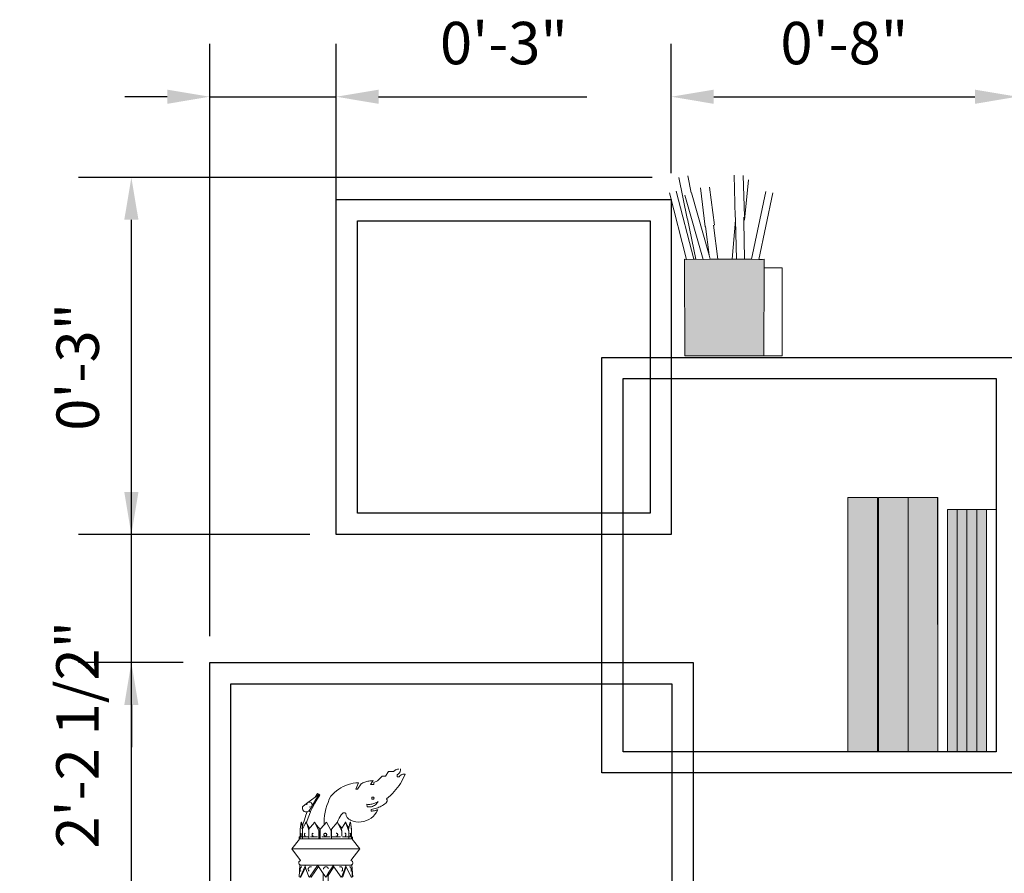
# Model space of a CAD drawing. Units: millimetres. Extents: x 7894 to 8038, y 6851 to 6951.
# Tile 6 of 49: x 7940.01 to 7963.22, y 6871.49 to 6891.62. Entities that reach past the tile are written whole.
import ezdxf

# ---------------------------------------------------------------- set-up
doc = ezdxf.new("R2010")
doc.units = ezdxf.units.MM
for name, color, linetype, lineweight in [('A-ANNO-DIMS', 2, 'Continuous', 18), ('A-FURN-ACCS', 8, 'Continuous', 13), ('A-FURN-BOOK', 8, 'Continuous', 13), ('A-FURN-CASE', 7, 'Continuous', 30)]:
    doc.layers.add(name, color=color, linetype=linetype, lineweight=lineweight)
doc.layers.add('A-FURN-ACCS-PATT', color=116, linetype='Continuous', lineweight=9, true_color=0x136734)
doc.layers.add('A-FURN-PATT', color=32, linetype='Continuous', lineweight=9, true_color=0xcd6928)
doc.styles.get("Standard").update_dxf_attribs({"font": 'arial.ttf'})
doc.dimstyles.new('ISO-25', dxfattribs={"dimtxt": 1, "dimasz": 1, "dimexe": 1.25, "dimexo": 0.625, "dimtad": 1, "dimdec": 0, "dimlunit": 4, "dimtxsty": 'Standard', "dimcen": 2.5, "dimclrt": 1, "dimadec": 0, "dimazin": 0, "dimtfac": 1, "dimtdec": 0, "dimtmove": 0, "dimatfit": 3, "dimfxl": 1, "dimarcsym": 0})

# ---------------------------------------------------------------- blocks, each defined once
blk = doc.blocks.new('DISPLAY-LEAF-FINIAL')
for p, q in [((2.447, 3.478), (2.461, 3.485)), ((2.461, 3.485), (2.475, 3.491)), ((2.475, 3.491), (2.489, 3.496)), ((2.489, 3.496), (2.504, 3.501)), ((2.504, 3.501), (2.519, 3.504)), ((2.565, 3.494), (2.563, 3.479)), ((2.565, 3.508), (2.565, 3.494)), ((2.023, 3.221), (2.127, 3.334)), ((2.127, 3.334), (2.209, 3.334)), ((2.209, 3.334), (2.276, 3.441)), ((2.276, 3.441), (2.398, 3.441)), ((2.398, 3.441), (2.409, 3.452)), ((2.409, 3.452), (2.421, 3.461)), ((2.421, 3.461), (2.434, 3.47)), ((2.434, 3.47), (2.447, 3.478)), ((2.493, 3.371), (2.48, 3.364)), ((2.48, 3.364), (2.48, 3.316)), ((2.48, 3.316), (2.533, 3.316)), ((2.505, 3.379), (2.493, 3.371)), ((2.516, 3.389), (2.505, 3.379)), ((2.527, 3.4), (2.516, 3.389)), ((2.536, 3.411), (2.527, 3.4)), ((2.533, 3.316), (2.54, 3.327)), ((2.544, 3.424), (2.536, 3.411)), ((2.54, 3.327), (2.549, 3.338)), ((2.551, 3.437), (2.544, 3.424)), ((2.549, 3.338), (2.558, 3.347)), ((2.556, 3.45), (2.551, 3.437)), ((2.56, 3.465), (2.556, 3.45)), ((2.558, 3.347), (2.569, 3.356)), ((2.563, 3.479), (2.56, 3.465)), ((2.569, 3.356), (2.58, 3.363)), ((2.58, 3.363), (2.592, 3.37)), ((2.62, 3.27), (2.591, 3.216)), ((2.592, 3.37), (2.604, 3.375)), ((2.604, 3.375), (2.617, 3.379)), ((2.617, 3.379), (2.63, 3.382)), ((2.646, 3.325), (2.62, 3.27)), ((2.63, 3.382), (2.643, 3.383)), ((2.643, 3.383), (2.657, 3.383)), ((2.67, 3.382), (2.646, 3.325)), ((2.657, 3.383), (2.67, 3.382)), ((1.055, 2.986), (1.105, 3.023)), ((1.105, 3.023), (1.158, 3.056)), ((1.158, 3.056), (1.213, 3.085)), ((1.213, 3.085), (1.27, 3.111)), ((1.27, 3.111), (1.328, 3.133)), ((1.328, 3.133), (1.388, 3.15)), ((1.388, 3.15), (1.449, 3.164)), ((1.449, 3.164), (1.51, 3.173)), ((1.51, 3.173), (1.572, 3.179)), ((1.572, 3.179), (1.511, 3.024)), ((1.511, 3.024), (1.55, 3.024)), ((1.55, 3.024), (1.632, 3.152)), ((1.632, 3.152), (1.654, 3.163)), ((1.654, 3.163), (1.676, 3.173)), ((1.676, 3.173), (1.699, 3.182)), ((1.699, 3.182), (1.722, 3.191)), ((1.722, 3.191), (1.745, 3.198)), ((1.745, 3.198), (1.769, 3.205)), ((1.769, 3.205), (1.793, 3.211)), ((1.793, 3.211), (1.817, 3.216)), ((1.817, 3.216), (1.841, 3.22)), ((1.841, 3.22), (1.865, 3.223)), ((1.914, 3.227), (1.854, 3.133)), ((1.854, 3.133), (1.934, 3.133)), ((1.865, 3.223), (1.889, 3.226)), ((1.889, 3.226), (1.914, 3.227)), ((1.934, 3.185), (2.023, 3.221)), ((1.934, 3.133), (1.934, 3.185)), ((2.491, 3.062), (2.453, 3.014)), ((2.527, 3.112), (2.491, 3.062)), ((2.56, 3.163), (2.527, 3.112)), ((2.591, 3.216), (2.56, 3.163)), ((0.547, 2.84), (0.379, 2.713)), ((0.634, 2.9), (0.463, 2.609)), ((0.541, 2.696), (0.599, 2.791)), ((0.605, 2.924), (0.547, 2.84)), ((0.634, 2.905), (0.547, 2.84)), ((0.599, 2.791), (0.663, 2.885)), ((0.634, 2.905), (0.605, 2.924)), ((0.634, 2.9), (0.634, 2.905)), ((0.663, 2.885), (0.634, 2.905)), ((0.884, 2.786), (0.853, 2.713)), ((0.92, 2.857), (0.884, 2.786)), ((0.92, 2.857), (0.962, 2.903)), ((0.962, 2.903), (1.007, 2.946)), ((1.007, 2.946), (1.055, 2.986)), ((1.883, 2.817), (1.885, 2.824)), ((1.883, 2.81), (1.883, 2.817)), ((1.885, 2.803), (1.883, 2.81)), ((1.885, 2.824), (1.889, 2.831)), ((1.888, 2.797), (1.885, 2.803)), ((1.894, 2.791), (1.888, 2.797)), ((1.889, 2.831), (1.894, 2.836)), ((1.894, 2.836), (1.9, 2.839)), ((1.9, 2.788), (1.894, 2.791)), ((1.9, 2.839), (1.907, 2.841)), ((1.907, 2.786), (1.9, 2.788)), ((1.907, 2.841), (1.914, 2.841)), ((1.914, 2.841), (1.921, 2.839)), ((1.921, 2.788), (1.914, 2.786)), ((1.921, 2.839), (1.928, 2.836)), ((1.928, 2.791), (1.921, 2.788)), ((1.928, 2.836), (1.933, 2.83)), ((1.933, 2.796), (1.928, 2.791)), ((1.933, 2.83), (1.937, 2.824)), ((1.936, 2.803), (1.933, 2.796)), ((1.938, 2.81), (1.936, 2.803)), ((1.937, 2.824), (1.938, 2.817)), ((1.938, 2.817), (1.938, 2.81)), ((2.281, 2.839), (2.233, 2.801)), ((2.233, 2.801), (2.238, 2.792)), ((2.238, 2.792), (2.242, 2.783)), ((2.327, 2.88), (2.281, 2.839)), ((2.371, 2.923), (2.327, 2.88)), ((2.413, 2.967), (2.371, 2.923)), ((2.453, 3.014), (2.413, 2.967)), ((0.253, 2.607), (0.249, 2.584)), ((0.249, 2.58), (0.249, 2.584)), ((0.249, 2.58), (0.251, 2.557)), ((0.251, 2.557), (0.259, 2.536)), ((0.264, 2.627), (0.253, 2.607)), ((0.379, 2.713), (0.264, 2.627)), ((0.353, 2.675), (0.358, 2.69)), ((0.353, 2.66), (0.353, 2.675)), ((0.353, 2.659), (0.353, 2.66)), ((0.353, 2.657), (0.353, 2.659)), ((0.358, 2.69), (0.367, 2.703)), ((0.367, 2.703), (0.379, 2.713)), ((0.379, 2.713), (0.393, 2.72)), ((0.393, 2.72), (0.409, 2.723)), ((0.409, 2.723), (0.425, 2.722)), ((0.414, 2.606), (0.413, 2.603)), ((0.461, 2.605), (0.415, 2.527)), ((0.425, 2.722), (0.44, 2.718)), ((0.44, 2.718), (0.453, 2.709)), ((0.44, 2.496), (0.486, 2.593)), ((0.443, 2.613), (0.446, 2.612)), ((0.451, 2.615), (0.449, 2.616)), ((0.453, 2.709), (0.464, 2.698)), ((0.463, 2.609), (0.461, 2.605)), ((0.486, 2.593), (0.461, 2.605)), ((0.463, 2.609), (0.488, 2.597)), ((0.464, 2.698), (0.471, 2.684)), ((0.471, 2.684), (0.475, 2.669)), ((0.474, 2.667), (0.475, 2.669)), ((0.474, 2.667), (0.475, 2.666)), ((0.541, 2.696), (0.488, 2.597)), ((0.804, 2.562), (0.787, 2.485)), ((0.826, 2.638), (0.804, 2.562)), ((0.853, 2.713), (0.826, 2.638)), ((1.793, 2.668), (1.77, 2.67)), ((1.77, 2.67), (1.776, 2.611)), ((1.801, 2.608), (1.776, 2.611)), ((1.816, 2.667), (1.793, 2.668)), ((1.827, 2.607), (1.801, 2.608)), ((1.84, 2.668), (1.816, 2.667)), ((1.852, 2.609), (1.827, 2.607)), ((1.863, 2.67), (1.84, 2.668)), ((1.878, 2.613), (1.852, 2.609)), ((1.886, 2.673), (1.863, 2.67)), ((1.902, 2.62), (1.878, 2.613)), ((1.909, 2.678), (1.886, 2.673)), ((1.926, 2.63), (1.902, 2.62)), ((1.934, 2.561), (1.903, 2.554)), ((1.914, 2.786), (1.907, 2.786)), ((1.931, 2.684), (1.909, 2.678)), ((1.949, 2.642), (1.926, 2.63)), ((1.954, 2.692), (1.931, 2.684)), ((1.964, 2.569), (1.934, 2.561)), ((1.97, 2.657), (1.949, 2.642)), ((1.975, 2.701), (1.954, 2.692)), ((1.994, 2.578), (1.964, 2.569)), ((1.99, 2.673), (1.97, 2.657)), ((1.996, 2.711), (1.975, 2.701)), ((2.007, 2.692), (1.99, 2.673)), ((2.024, 2.588), (1.994, 2.578)), ((2.017, 2.722), (1.996, 2.711)), ((2.023, 2.712), (2.007, 2.692)), ((2.036, 2.734), (2.017, 2.722)), ((2.036, 2.734), (2.023, 2.712)), ((2.053, 2.6), (2.024, 2.588)), ((2.082, 2.613), (2.053, 2.6)), ((2.11, 2.627), (2.082, 2.613)), ((2.137, 2.643), (2.11, 2.627)), ((2.164, 2.659), (2.137, 2.643)), ((2.19, 2.677), (2.164, 2.659)), ((2.216, 2.695), (2.19, 2.677)), ((2.223, 2.702), (2.216, 2.695)), ((2.23, 2.709), (2.223, 2.702)), ((2.235, 2.717), (2.23, 2.709)), ((2.24, 2.726), (2.235, 2.717)), ((2.243, 2.735), (2.24, 2.726)), ((2.242, 2.783), (2.245, 2.774)), ((2.245, 2.745), (2.243, 2.735)), ((2.245, 2.774), (2.246, 2.764)), ((2.246, 2.754), (2.245, 2.745)), ((2.246, 2.764), (2.246, 2.754)), ((0.259, 2.536), (0.272, 2.517)), ((0.272, 2.517), (0.29, 2.502)), ((0.29, 2.502), (0.311, 2.492)), ((0.332, 2.415), (0.295, 2.306)), ((0.311, 2.492), (0.334, 2.488)), ((0.363, 2.491), (0.332, 2.415)), ((0.334, 2.488), (0.358, 2.489)), ((0.358, 2.489), (0.363, 2.491)), ((0.361, 2.285), (0.398, 2.391)), ((0.363, 2.491), (0.38, 2.497)), ((0.365, 2.496), (0.363, 2.491)), ((0.38, 2.497), (0.4, 2.51)), ((0.398, 2.513), (0.402, 2.512)), ((0.398, 2.391), (0.44, 2.495)), ((0.403, 2.513), (0.4, 2.514)), ((0.4, 2.51), (0.402, 2.512)), ((0.402, 2.512), (0.403, 2.513)), ((0.402, 2.512), (0.44, 2.495)), ((0.403, 2.513), (0.415, 2.527)), ((0.403, 2.513), (0.44, 2.496)), ((0.409, 2.511), (0.408, 2.509)), ((0.42, 2.535), (0.409, 2.511)), ((0.766, 2.327), (0.763, 2.248)), ((0.774, 2.406), (0.766, 2.327)), ((0.787, 2.485), (0.774, 2.406)), ((1.113, 2.339), (1.092, 2.297)), ((1.136, 2.379), (1.113, 2.339)), ((1.163, 2.417), (1.136, 2.379)), ((1.193, 2.452), (1.163, 2.417)), ((1.198, 2.457), (1.193, 2.452)), ((1.204, 2.462), (1.198, 2.457)), ((1.211, 2.465), (1.204, 2.462)), ((1.218, 2.467), (1.211, 2.465)), ((1.225, 2.469), (1.218, 2.467)), ((1.232, 2.47), (1.225, 2.469)), ((1.239, 2.469), (1.232, 2.47)), ((1.247, 2.467), (1.239, 2.469)), ((1.254, 2.465), (1.247, 2.467)), ((1.26, 2.462), (1.254, 2.465)), ((1.266, 2.457), (1.26, 2.462)), ((1.271, 2.452), (1.266, 2.457)), ((1.274, 2.435), (1.271, 2.452)), ((1.278, 2.418), (1.274, 2.435)), ((1.283, 2.402), (1.278, 2.418)), ((1.29, 2.386), (1.283, 2.402)), ((1.298, 2.371), (1.29, 2.386)), ((1.308, 2.357), (1.298, 2.371)), ((1.319, 2.343), (1.308, 2.357)), ((1.331, 2.331), (1.319, 2.343)), ((1.343, 2.319), (1.331, 2.331)), ((1.87, 2.344), (1.816, 2.31)), ((1.918, 2.385), (1.87, 2.344)), ((1.903, 2.554), (1.872, 2.548)), ((1.872, 2.548), (1.872, 2.508)), ((1.872, 2.508), (1.885, 2.509)), ((1.885, 2.509), (1.898, 2.51)), ((1.898, 2.51), (1.911, 2.511)), ((1.911, 2.511), (1.924, 2.513)), ((1.961, 2.432), (1.918, 2.385)), ((1.924, 2.513), (1.937, 2.515)), ((1.937, 2.515), (1.95, 2.518)), ((1.95, 2.518), (1.963, 2.521)), ((1.997, 2.484), (1.961, 2.432)), ((1.963, 2.521), (1.976, 2.524)), ((1.976, 2.524), (1.988, 2.528)), ((1.988, 2.528), (2.001, 2.532)), ((2.026, 2.541), (1.997, 2.484)), ((2.001, 2.532), (2.013, 2.536)), ((2.013, 2.536), (2.026, 2.541)), ((0.213, 2.19), (0.195, 2.086)), ((0.213, 2.19), (0.215, 2.201)), ((0.215, 2.201), (0.22, 2.245)), ((0.223, 2.245), (0.215, 2.201)), ((0.223, 2.245), (0.22, 2.245)), ((0.223, 2.245), (0.23, 2.245)), ((0.232, 2.22), (0.23, 2.245)), ((0.232, 2.22), (0.25, 2.138)), ((0.244, 2.11), (0.232, 2.22)), ((0.244, 2.11), (0.239, 2.089)), ((0.25, 2.138), (0.244, 2.11)), ((0.248, 2.065), (0.244, 2.11)), ((0.317, 2.207), (0.248, 2.086)), ((0.263, 2.194), (0.25, 2.138)), ((0.25, 2.138), (0.256, 2.115)), ((0.295, 2.306), (0.263, 2.194)), ((0.297, 2.185), (0.292, 2.162)), ((0.317, 2.207), (0.33, 2.245)), ((0.338, 2.245), (0.317, 2.207)), ((0.332, 2.245), (0.33, 2.245)), ((0.344, 2.245), (0.338, 2.245)), ((0.347, 2.235), (0.344, 2.245)), ((0.347, 2.235), (0.361, 2.285)), ((0.354, 2.213), (0.347, 2.235)), ((0.354, 2.213), (0.42, 2.104)), ((0.404, 2.061), (0.354, 2.213)), ((0.42, 2.104), (0.404, 2.086)), ((0.507, 2.209), (0.42, 2.104)), ((0.507, 2.209), (0.525, 2.245)), ((0.532, 2.239), (0.507, 2.209)), ((0.528, 2.245), (0.525, 2.245)), ((0.528, 2.245), (0.532, 2.239)), ((0.537, 2.245), (0.532, 2.239)), ((0.54, 2.245), (0.537, 2.245)), ((0.556, 2.211), (0.54, 2.245)), ((0.548, 2.22), (0.556, 2.211)), ((0.556, 2.211), (0.663, 2.086)), ((0.636, 2.045), (0.556, 2.211)), ((0.765, 2.186), (0.671, 2.086)), ((0.763, 2.248), (0.765, 2.186)), ((0.821, 2.245), (0.765, 2.186)), ((0.93, 2.045), (0.821, 2.245)), ((1.07, 2.239), (0.939, 2.086)), ((1.07, 2.239), (1.069, 2.235)), ((1.071, 2.24), (1.07, 2.239)), ((1.07, 2.239), (1.071, 2.237)), ((1.075, 2.254), (1.071, 2.24)), ((1.074, 2.245), (1.071, 2.24)), ((1.074, 2.245), (1.078, 2.245)), ((1.092, 2.297), (1.075, 2.254)), ((1.095, 2.209), (1.078, 2.245)), ((1.095, 2.209), (1.182, 2.104)), ((1.095, 2.209), (1.171, 2.054)), ((1.182, 2.104), (1.171, 2.086)), ((1.248, 2.213), (1.182, 2.104)), ((1.248, 2.213), (1.258, 2.245)), ((1.265, 2.242), (1.248, 2.213)), ((1.258, 2.245), (1.264, 2.245)), ((1.264, 2.245), (1.265, 2.242)), ((1.267, 2.245), (1.265, 2.242)), ((1.267, 2.245), (1.272, 2.245)), ((1.285, 2.207), (1.272, 2.245)), ((1.285, 2.207), (1.344, 2.103)), ((1.285, 2.207), (1.34, 2.048)), ((1.344, 2.103), (1.34, 2.086)), ((1.357, 2.309), (1.343, 2.319)), ((1.37, 2.22), (1.344, 2.103)), ((1.372, 2.3), (1.357, 2.309)), ((1.37, 2.22), (1.372, 2.245)), ((1.375, 2.245), (1.37, 2.22)), ((1.387, 2.292), (1.372, 2.3)), ((1.372, 2.245), (1.375, 2.245)), ((1.375, 2.245), (1.382, 2.245)), ((1.382, 2.245), (1.389, 2.19)), ((1.447, 2.27), (1.387, 2.292)), ((1.389, 2.19), (1.408, 2.086)), ((1.407, 2.045), (1.389, 2.19)), ((1.509, 2.256), (1.447, 2.27)), ((1.572, 2.25), (1.509, 2.256)), ((1.635, 2.253), (1.572, 2.25)), ((1.698, 2.264), (1.635, 2.253)), ((1.759, 2.283), (1.698, 2.264)), ((1.816, 2.31), (1.759, 2.283)), ((0.17, 1.877), (0.172, 1.885)), ((0.17, 1.87), (0.17, 1.877)), ((0.172, 1.862), (0.17, 1.87)), ((0.172, 1.885), (0.176, 1.892)), ((0.175, 1.855), (0.172, 1.862)), ((0.176, 1.892), (0.182, 1.898)), ((0.182, 1.898), (0.189, 1.901)), ((0.189, 1.901), (0.195, 1.903)), ((0.195, 2.086), (0.195, 2.048)), ((0.195, 2.045), (0.195, 2.048)), ((0.195, 2.045), (0.195, 1.903)), ((0.195, 1.903), (0.195, 1.901)), ((0.195, 1.903), (0.196, 1.903)), ((0.195, 1.898), (0.195, 1.87)), ((0.195, 1.862), (0.195, 1.855)), ((0.196, 1.903), (0.198, 1.903)), ((0.196, 1.903), (0.197, 1.903)), ((0.237, 1.903), (0.198, 1.903)), ((0.207, 1.965), (0.208, 1.973)), ((0.207, 1.956), (0.207, 1.965)), ((0.207, 1.947), (0.207, 1.956)), ((0.207, 1.938), (0.207, 1.947)), ((0.208, 1.93), (0.207, 1.938)), ((0.208, 1.973), (0.209, 1.979)), ((0.209, 1.924), (0.208, 1.93)), ((0.209, 1.979), (0.211, 1.984)), ((0.211, 1.919), (0.209, 1.924)), ((0.21, 1.956), (0.211, 1.965)), ((0.21, 1.947), (0.21, 1.956)), ((0.211, 1.938), (0.21, 1.947)), ((0.211, 1.984), (0.213, 1.986)), ((0.211, 1.965), (0.212, 1.973)), ((0.212, 1.93), (0.211, 1.938)), ((0.213, 1.917), (0.211, 1.919)), ((0.212, 1.973), (0.213, 1.979)), ((0.213, 1.924), (0.212, 1.93)), ((0.216, 1.986), (0.213, 1.986)), ((0.213, 1.979), (0.214, 1.984)), ((0.216, 1.947), (0.213, 1.924)), ((0.214, 1.919), (0.213, 1.924)), ((0.214, 1.917), (0.213, 1.917)), ((0.214, 1.984), (0.216, 1.986)), ((0.216, 1.917), (0.214, 1.919)), ((0.216, 1.917), (0.214, 1.917)), ((0.217, 1.965), (0.216, 1.956)), ((0.216, 1.956), (0.216, 1.947)), ((0.216, 1.947), (0.217, 1.938)), ((0.218, 1.917), (0.216, 1.917)), ((0.218, 1.973), (0.217, 1.965)), ((0.218, 1.967), (0.217, 1.965)), ((0.217, 1.938), (0.218, 1.93)), ((0.219, 1.979), (0.218, 1.973)), ((0.218, 1.973), (0.218, 1.967)), ((0.218, 1.93), (0.219, 1.924)), ((0.22, 1.981), (0.219, 1.979)), ((0.22, 1.981), (0.219, 1.979)), ((0.219, 1.924), (0.22, 1.921)), ((0.221, 1.973), (0.22, 1.965)), ((0.22, 1.965), (0.22, 1.956)), ((0.22, 1.956), (0.22, 1.947)), ((0.22, 1.947), (0.22, 1.938)), ((0.22, 1.938), (0.221, 1.93)), ((0.222, 1.975), (0.221, 1.973)), ((0.221, 1.93), (0.222, 1.928)), ((0.248, 1.903), (0.244, 1.903)), ((0.245, 1.898), (0.244, 1.886)), ((0.248, 1.897), (0.244, 1.897)), ((0.248, 1.925), (0.246, 1.901)), ((0.248, 2.086), (0.248, 2.065)), ((0.248, 2.065), (0.248, 1.903)), ((0.248, 1.903), (0.248, 1.901)), ((0.248, 1.898), (0.248, 1.897)), ((0.248, 1.897), (0.248, 1.87)), ((0.248, 1.862), (0.248, 1.855)), ((0.391, 1.903), (0.265, 1.903)), ((0.295, 1.956), (0.297, 1.965)), ((0.295, 1.947), (0.295, 1.956)), ((0.297, 1.938), (0.295, 1.947)), ((0.297, 1.965), (0.3, 1.973)), ((0.3, 1.93), (0.297, 1.938)), ((0.3, 1.973), (0.304, 1.979)), ((0.303, 1.924), (0.3, 1.93)), ((0.308, 1.919), (0.303, 1.924)), ((0.304, 1.979), (0.308, 1.984)), ((0.308, 1.984), (0.314, 1.986)), ((0.313, 1.917), (0.308, 1.919)), ((0.319, 1.917), (0.313, 1.917)), ((0.316, 1.986), (0.314, 1.986)), ((0.322, 1.917), (0.319, 1.917)), ((0.404, 2.086), (0.404, 2.061)), ((0.404, 2.061), (0.404, 1.901)), ((0.404, 1.898), (0.404, 1.87)), ((0.404, 1.862), (0.405, 1.855)), ((0.439, 1.903), (0.607, 1.903)), ((0.476, 1.956), (0.478, 1.965)), ((0.476, 1.947), (0.476, 1.956)), ((0.478, 1.938), (0.476, 1.947)), ((0.478, 1.965), (0.482, 1.973)), ((0.482, 1.93), (0.478, 1.938)), ((0.482, 1.973), (0.488, 1.979)), ((0.488, 1.924), (0.482, 1.93)), ((0.488, 1.979), (0.495, 1.984)), ((0.495, 1.919), (0.488, 1.924)), ((0.495, 1.984), (0.502, 1.986)), ((0.502, 1.917), (0.495, 1.919)), ((0.504, 1.986), (0.502, 1.986)), ((0.51, 1.917), (0.502, 1.917)), ((0.512, 1.917), (0.51, 1.917)), ((0.637, 1.903), (0.634, 1.903)), ((0.637, 1.897), (0.634, 1.897)), ((0.636, 2.045), (0.637, 1.903)), ((0.637, 1.903), (0.637, 1.901)), ((0.663, 1.903), (0.637, 1.903)), ((0.637, 1.898), (0.637, 1.897)), ((0.637, 1.897), (0.637, 1.87)), ((0.663, 1.897), (0.637, 1.897)), ((0.637, 1.862), (0.637, 1.855)), ((0.663, 2.086), (0.663, 1.903)), ((0.663, 1.903), (0.671, 1.903)), ((0.663, 1.903), (0.663, 1.901)), ((0.663, 1.898), (0.663, 1.897)), ((0.663, 1.897), (0.663, 1.87)), ((0.671, 1.897), (0.663, 1.897)), ((0.663, 1.862), (0.663, 1.855)), ((0.671, 2.086), (0.671, 1.903)), ((0.671, 1.903), (0.671, 1.901)), ((0.671, 1.898), (0.671, 1.897)), ((0.671, 1.897), (0.671, 1.87)), ((0.671, 1.862), (0.671, 1.855)), ((0.708, 1.903), (0.894, 1.903)), ((0.754, 1.956), (0.756, 1.965)), ((0.754, 1.947), (0.754, 1.956)), ((0.756, 1.938), (0.754, 1.947)), ((0.756, 1.965), (0.761, 1.973)), ((0.761, 1.93), (0.756, 1.938)), ((0.761, 1.973), (0.767, 1.979)), ((0.767, 1.924), (0.761, 1.93)), ((0.767, 1.979), (0.775, 1.984)), ((0.775, 1.919), (0.767, 1.924)), ((0.775, 1.984), (0.784, 1.986)), ((0.784, 1.917), (0.775, 1.919)), ((0.784, 1.986), (0.793, 1.986)), ((0.793, 1.917), (0.784, 1.917)), ((0.793, 1.986), (0.802, 1.984)), ((0.802, 1.919), (0.793, 1.917)), ((0.802, 1.984), (0.81, 1.979)), ((0.81, 1.924), (0.802, 1.919)), ((0.81, 1.979), (0.816, 1.973)), ((0.816, 1.93), (0.81, 1.924)), ((0.816, 1.973), (0.821, 1.965)), ((0.821, 1.938), (0.816, 1.93)), ((0.821, 1.965), (0.823, 1.956)), ((0.823, 1.947), (0.821, 1.938)), ((0.823, 1.956), (0.823, 1.947)), ((0.93, 2.045), (0.931, 1.934)), ((0.939, 1.934), (0.931, 1.934)), ((0.931, 1.934), (0.931, 1.903)), ((0.931, 1.903), (0.931, 1.901)), ((0.939, 1.903), (0.931, 1.903)), ((0.931, 1.898), (0.931, 1.897)), ((0.931, 1.897), (0.932, 1.87)), ((0.939, 1.897), (0.931, 1.897)), ((0.932, 1.862), (0.932, 1.855)), ((0.939, 2.086), (0.939, 1.934)), ((0.942, 1.934), (0.939, 1.934)), ((0.939, 1.934), (0.939, 1.903)), ((0.942, 1.903), (0.939, 1.903)), ((0.939, 1.903), (0.939, 1.901)), ((0.939, 1.898), (0.939, 1.897)), ((0.942, 1.897), (0.939, 1.897)), ((0.939, 1.897), (0.939, 1.87)), ((0.939, 1.862), (0.939, 1.855)), ((0.953, 1.903), (1.146, 1.903)), ((1.022, 1.935), (1.021, 1.935)), ((1.044, 1.986), (1.046, 1.986)), ((1.046, 1.986), (1.054, 1.986)), ((1.052, 1.917), (1.054, 1.917)), ((1.054, 1.986), (1.062, 1.984)), ((1.062, 1.919), (1.054, 1.917)), ((1.062, 1.984), (1.069, 1.979)), ((1.069, 1.924), (1.062, 1.919)), ((1.069, 1.979), (1.075, 1.973)), ((1.075, 1.93), (1.069, 1.924)), ((1.075, 1.973), (1.079, 1.965)), ((1.079, 1.938), (1.075, 1.93)), ((1.079, 1.965), (1.081, 1.956)), ((1.081, 1.947), (1.079, 1.938)), ((1.081, 1.956), (1.081, 1.947)), ((1.171, 2.086), (1.171, 2.054)), ((1.176, 2.045), (1.171, 2.054)), ((1.176, 2.045), (1.177, 1.914)), ((1.33, 1.903), (1.197, 1.903)), ((1.249, 1.986), (1.251, 1.986)), ((1.251, 1.986), (1.257, 1.986)), ((1.254, 1.917), (1.257, 1.917)), ((1.257, 1.986), (1.263, 1.984)), ((1.263, 1.919), (1.257, 1.917)), ((1.263, 1.984), (1.268, 1.979)), ((1.268, 1.924), (1.263, 1.919)), ((1.268, 1.979), (1.272, 1.973)), ((1.272, 1.93), (1.268, 1.924)), ((1.272, 1.973), (1.275, 1.965)), ((1.275, 1.938), (1.272, 1.93)), ((1.275, 1.965), (1.276, 1.956)), ((1.276, 1.947), (1.275, 1.938)), ((1.276, 1.956), (1.276, 1.947)), ((1.34, 2.086), (1.34, 2.048)), ((1.341, 2.045), (1.34, 2.048)), ((1.341, 2.045), (1.342, 1.903)), ((1.347, 1.903), (1.342, 1.903)), ((1.342, 1.903), (1.342, 1.901)), ((1.342, 1.898), (1.342, 1.897)), ((1.347, 1.897), (1.342, 1.897)), ((1.342, 1.897), (1.342, 1.87)), ((1.342, 1.862), (1.342, 1.855)), ((1.356, 1.903), (1.4, 1.903)), ((1.373, 1.986), (1.376, 1.986)), ((1.378, 1.919), (1.375, 1.917)), ((1.375, 1.917), (1.379, 1.917)), ((1.376, 1.986), (1.378, 1.984)), ((1.376, 1.986), (1.377, 1.986)), ((1.377, 1.986), (1.379, 1.986)), ((1.378, 1.984), (1.379, 1.979)), ((1.379, 1.924), (1.378, 1.919)), ((1.379, 1.986), (1.381, 1.984)), ((1.379, 1.979), (1.381, 1.973)), ((1.381, 1.93), (1.379, 1.924)), ((1.381, 1.919), (1.379, 1.917)), ((1.381, 1.984), (1.383, 1.979)), ((1.381, 1.973), (1.382, 1.965)), ((1.382, 1.938), (1.381, 1.93)), ((1.383, 1.924), (1.381, 1.919)), ((1.382, 1.965), (1.382, 1.956)), ((1.382, 1.956), (1.382, 1.947)), ((1.382, 1.947), (1.382, 1.938)), ((1.383, 1.979), (1.384, 1.973)), ((1.384, 1.93), (1.383, 1.924)), ((1.384, 1.973), (1.385, 1.965)), ((1.385, 1.938), (1.384, 1.93)), ((1.385, 1.965), (1.386, 1.956)), ((1.386, 1.947), (1.385, 1.938)), ((1.386, 1.956), (1.386, 1.947)), ((1.408, 2.086), (1.407, 2.045)), ((1.407, 2.045), (1.408, 1.903)), ((1.408, 1.903), (1.413, 1.901)), ((1.408, 1.903), (1.408, 1.901)), ((1.408, 1.898), (1.408, 1.87)), ((1.408, 1.862), (1.408, 1.855)), ((1.413, 1.901), (1.42, 1.898)), ((1.42, 1.898), (1.426, 1.892)), ((1.426, 1.892), (1.43, 1.885)), ((1.431, 1.862), (1.427, 1.855)), ((1.43, 1.885), (1.432, 1.877)), ((1.433, 1.87), (1.431, 1.862)), ((1.432, 1.877), (1.433, 1.87)), ((0, 1.62), (0.181, 1.849)), ((0.181, 1.849), (0.175, 1.855)), ((0.195, 1.855), (0.195, 1.855)), ((0.205, 1.855), (0.195, 1.855)), ((0.205, 1.855), (0.205, 1.851)), ((0.248, 1.855), (0.205, 1.855)), ((0.205, 1.851), (0.205, 1.849)), ((0.24, 1.855), (0.24, 1.849)), ((0.248, 1.855), (0.276, 1.855)), ((0.275, 1.849), (0.276, 1.855)), ((0.276, 1.855), (0.405, 1.855)), ((0.405, 1.855), (0.637, 1.855)), ((0.663, 1.855), (0.637, 1.855)), ((0.671, 1.855), (0.932, 1.855)), ((0.939, 1.855), (0.932, 1.855)), ((1.342, 1.855), (0.939, 1.855)), ((1.408, 1.855), (1.342, 1.855)), ((1.427, 1.855), (1.421, 1.849)), ((1.421, 1.849), (1.602, 1.62)), ((0.207, 1.343), (0, 1.62)), ((1.602, 1.62), (0, 1.62)), ((1.602, 1.62), (1.395, 1.343)), ((0.164, 1.297), (0.168, 1.31)), ((0.164, 1.283), (0.164, 1.297)), ((0.167, 1.27), (0.164, 1.283)), ((0.173, 1.258), (0.167, 1.27)), ((0.168, 1.31), (0.174, 1.321)), ((0.171, 0.955), (0.191, 1.234)), ((0.182, 1.248), (0.173, 1.258)), ((0.174, 1.321), (0.183, 1.331)), ((0.193, 1.24), (0.182, 1.248)), ((0.183, 1.331), (0.195, 1.338)), ((0.219, 1.234), (0.191, 1.234)), ((0.206, 1.236), (0.193, 1.24)), ((0.195, 1.338), (0.207, 1.343)), ((0.196, 0.954), (0.311, 1.21)), ((0.202, 1.152), (0.206, 1.165)), ((0.219, 1.234), (0.206, 1.236)), ((0.206, 1.165), (0.212, 1.177)), ((0.212, 1.177), (0.217, 1.187)), ((0.215, 0.949), (0.324, 1.172)), ((0.217, 1.187), (0.223, 1.193)), ((0.219, 1.234), (0.297, 1.234)), ((0.223, 1.193), (0.228, 1.197)), ((0.228, 1.197), (0.232, 1.196)), ((0.232, 1.195), (0.232, 1.196)), ((0.232, 1.195), (0.237, 1.195)), ((0.297, 1.234), (0.302, 1.234)), ((0.303, 1.232), (0.297, 1.234)), ((0.303, 1.232), (0.302, 1.234)), ((0.302, 1.234), (0.594, 1.234)), ((0.311, 1.21), (0.303, 1.232)), ((0.324, 1.172), (0.311, 1.21)), ((0.402, 0.955), (0.324, 1.172)), ((0.389, 1.152), (0.395, 1.165)), ((0.395, 1.165), (0.403, 1.177)), ((0.403, 1.177), (0.413, 1.187)), ((0.413, 1.187), (0.424, 1.193)), ((0.424, 1.193), (0.436, 1.197)), ((0.434, 0.975), (0.609, 1.228)), ((0.436, 1.197), (0.448, 1.196)), ((0.448, 1.196), (0.458, 1.192)), ((0.455, 0.949), (0.632, 1.205)), ((0.458, 1.192), (0.461, 1.191)), ((0.594, 1.234), (0.617, 1.234)), ((0.609, 1.228), (0.594, 1.234)), ((0.617, 1.228), (0.617, 1.234)), ((0.952, 1.234), (0.617, 1.234)), ((0.632, 1.205), (0.617, 1.228)), ((0.742, 1.037), (0.632, 1.205)), ((0.748, 1.152), (0.752, 1.165)), ((0.752, 1.165), (0.76, 1.177)), ((0.76, 1.177), (0.77, 1.187)), ((0.77, 1.187), (0.783, 1.193)), ((0.783, 1.193), (0.797, 1.197)), ((0.797, 1.197), (0.812, 1.196)), ((0.812, 1.196), (0.826, 1.192)), ((0.826, 1.192), (0.838, 1.185)), ((0.838, 1.185), (0.848, 1.175)), ((0.848, 1.175), (0.855, 1.162)), ((0.855, 1.162), (0.859, 1.148)), ((0.86, 1.041), (0.977, 1.215)), ((0.86, 0.992), (0.99, 1.195)), ((0.981, 1.234), (0.952, 1.234)), ((0.977, 1.215), (0.974, 1.218)), ((0.99, 1.195), (0.977, 1.215)), ((0.981, 1.234), (0.982, 1.234)), ((0.982, 1.234), (0.983, 1.234)), ((1.284, 1.234), (0.983, 1.234)), ((1.16, 0.949), (0.99, 1.195)), ((1.124, 1.192), (1.126, 1.193)), ((1.126, 1.193), (1.127, 1.193)), ((1.127, 1.193), (1.138, 1.197)), ((1.138, 1.197), (1.15, 1.196)), ((1.15, 1.196), (1.162, 1.192)), ((1.162, 1.192), (1.174, 1.185)), ((1.174, 1.185), (1.184, 1.175)), ((1.177, 0.964), (1.275, 1.212)), ((1.184, 1.175), (1.191, 1.162)), ((1.191, 1.162), (1.196, 1.148)), ((1.202, 0.955), (1.285, 1.19)), ((1.275, 1.212), (1.283, 1.232)), ((1.285, 1.19), (1.275, 1.212)), ((1.283, 1.232), (1.29, 1.234)), ((1.283, 1.232), (1.284, 1.234)), ((1.284, 1.234), (1.29, 1.234)), ((1.398, 0.949), (1.285, 1.19)), ((1.29, 1.234), (1.383, 1.234)), ((1.359, 1.195), (1.364, 1.197)), ((1.359, 1.195), (1.362, 1.195)), ((1.364, 1.197), (1.369, 1.196)), ((1.369, 1.196), (1.374, 1.192)), ((1.374, 1.192), (1.38, 1.185)), ((1.38, 1.185), (1.386, 1.175)), ((1.397, 1.236), (1.383, 1.234)), ((1.41, 1.234), (1.383, 1.234)), ((1.386, 1.175), (1.392, 1.162)), ((1.392, 1.162), (1.396, 1.148)), ((1.395, 1.343), (1.408, 1.338)), ((1.409, 1.24), (1.397, 1.236)), ((1.408, 1.338), (1.419, 1.331)), ((1.42, 1.248), (1.409, 1.24)), ((1.411, 1.234), (1.41, 1.234)), ((1.411, 1.232), (1.411, 1.234)), ((1.435, 0.955), (1.411, 1.232)), ((1.42, 0.955), (1.411, 1.232)), ((1.419, 1.331), (1.428, 1.321)), ((1.429, 1.258), (1.42, 1.248)), ((1.428, 1.321), (1.434, 1.31)), ((1.435, 1.27), (1.429, 1.258)), ((1.434, 1.31), (1.438, 1.297)), ((1.438, 1.283), (1.435, 1.27)), ((1.438, 1.297), (1.438, 1.283)), ((0.194, 0.949), (0.171, 0.955)), ((0.194, 1.111), (0.196, 1.124)), ((0.195, 1.101), (0.194, 1.111)), ((0.194, 0.949), (0.196, 0.954)), ((0.196, 1.094), (0.195, 1.101)), ((0.196, 1.124), (0.198, 1.137)), ((0.199, 1.09), (0.196, 1.094)), ((0.215, 0.949), (0.196, 0.954)), ((0.198, 1.137), (0.202, 1.152)), ((0.203, 1.089), (0.199, 1.09)), ((0.204, 1.088), (0.203, 1.089)), ((0.211, 1.096), (0.213, 1.092)), ((0.213, 1.092), (0.214, 1.092)), ((0.214, 1.1), (0.214, 1.098)), ((0.387, 1.137), (0.389, 1.152)), ((0.387, 1.124), (0.387, 1.137)), ((0.391, 1.111), (0.387, 1.124)), ((0.397, 1.101), (0.391, 1.111)), ((0.406, 1.094), (0.397, 1.101)), ((0.416, 0.949), (0.402, 0.955)), ((0.409, 1.092), (0.406, 1.094)), ((0.416, 0.949), (0.434, 0.975)), ((0.442, 0.955), (0.434, 0.975)), ((0.455, 0.949), (0.442, 0.955)), ((0.742, 0), (0.742, 1.037)), ((0.799, 0.949), (0.742, 1.037)), ((0.747, 1.137), (0.748, 1.152)), ((0.747, 1.136), (0.747, 1.137)), ((0.799, 0.949), (0.816, 0.974)), ((0.816, 0.974), (0.814, 0.977)), ((0.816, 0.974), (0.86, 1.041)), ((0.816, 0.973), (0.816, 0.974)), ((0.843, 0.965), (0.86, 0.992)), ((0.859, 1.147), (0.859, 1.148)), ((0.86, 1.041), (0.86, 1.047)), ((0.86, 0.992), (0.86, 1.041)), ((0.86, 0), (0.86, 0.992)), ((1.16, 0.949), (1.173, 0.955)), ((1.174, 1.092), (1.172, 1.091)), ((1.173, 0.955), (1.177, 0.964)), ((1.174, 1.092), (1.175, 1.092)), ((1.185, 1.099), (1.175, 1.092)), ((1.187, 0.949), (1.177, 0.964)), ((1.192, 1.109), (1.185, 1.099)), ((1.187, 0.949), (1.202, 0.955)), ((1.196, 1.121), (1.192, 1.109)), ((1.196, 1.148), (1.198, 1.134)), ((1.198, 1.134), (1.196, 1.121)), ((1.392, 1.089), (1.39, 1.088)), ((1.39, 1.088), (1.395, 1.089)), ((1.399, 1.092), (1.395, 1.089)), ((1.396, 1.148), (1.4, 1.134)), ((1.398, 0.949), (1.41, 0.953)), ((1.401, 1.099), (1.399, 1.092)), ((1.4, 1.134), (1.402, 1.121)), ((1.402, 1.109), (1.401, 1.099)), ((1.402, 1.121), (1.402, 1.109)), ((1.41, 0.953), (1.42, 0.955)), ((1.412, 0.949), (1.41, 0.953)), ((1.412, 0.949), (1.435, 0.955))]:
    blk.add_line(p, q)
blk = doc.blocks.new('DISPLAY-REED-SPRAY')
for p, q in [((0.218, 1.934), (0.42, 0.963)), ((0.515, 1.573), (0.435, 1.972)), ((1.548, 0.994), (1.529, 1.989)), ((1.766, 1.01), (1.742, 1.98)), ((1.77, 0.926), (1.861, 1.878)), ((0.846, 0.767), (0.729, 1.689)), ((1.062, 0.811), (0.945, 1.707)), ((0, 1.572), (0.406, 0.001)), ((0.578, 0.003), (0.162, 1.611)), ((0.792, 0), (0.361, 1.519)), ((0.935, 0.103), (0.519, 1.567)), ((1.938, 0.003), (2.275, 1.603)), ((2.108, 0.001), (2.44, 1.573)), ((0.62, 0.003), (0.428, 0.96)), ((1.56, 0.991), (1.561, 0.935)), ((1.56, 0.927), (1.561, 0.935)), ((1.753, 0.892), (1.751, 0.999)), ((0.935, 0.103), (0.852, 0.78)), ((1.139, 0.003), (1.042, 0.808)), ((1.477, 0.003), (1.56, 0.927)), ((1.56, 0.927), (1.58, 0.003)), ((1.753, 0.892), (1.755, 0.914)), ((1.771, 0.003), (1.753, 0.892)), ((0.963, 0.002), (0.935, 0.103))]:
    blk.add_line(p, q)
blk = doc.blocks.new('*D36')
at = {"layer": 'A-ANNO-DIMS', "color": 0, "lineweight": -2, "transparency": 16777216}
for p, q in [((7980.836, 6877.959), (7980.836, 6858.512)), ((7944.487, 6864.436), (7944.487, 6858.512)), ((7945.487, 6859.762), (7979.836, 6859.762))]:
    blk.add_line(p, q, dxfattribs=at)
at = {"layer": 'A-ANNO-DIMS', "color": 0, "transparency": 16777216}
for points in [[(7945.487, 6859.929), (7945.487, 6859.596), (7944.487, 6859.762)], [(7979.836, 6859.929), (7979.836, 6859.596), (7980.836, 6859.762)]]:
    blk.add_solid(points, dxfattribs=at)
at = {"layer": 'Defpoints', "color": 0, "transparency": 16777216}
for p in [(7980.836, 6878.584), (7944.487, 6865.061), (7980.836, 6859.762)]:
    blk.add_point(p, dxfattribs=at)
at = {"layer": 'A-ANNO-DIMS', "color": 1, "transparency": 16777216, "insert": (7962.661, 6860.905), "char_height": 1, "attachment_point": 5}
blk.add_mtext('3\'-0 1/2"', dxfattribs=at)
blk = doc.blocks.new('*D37')
at = {"layer": 'A-ANNO-DIMS', "color": 0, "lineweight": -2, "transparency": 16777216}
for p, q in [((7954.92, 6887.903), (7941.389, 6887.903)), ((7942.639, 6862.61), (7942.639, 6886.903)), ((7953.623, 6861.61), (7941.389, 6861.61))]:
    blk.add_line(p, q, dxfattribs=at)
at = {"layer": 'A-ANNO-DIMS', "color": 0, "transparency": 16777216}
for points in [[(7942.472, 6886.903), (7942.806, 6886.903), (7942.639, 6887.903)], [(7942.472, 6862.61), (7942.806, 6862.61), (7942.639, 6861.61)]]:
    blk.add_solid(points, dxfattribs=at)
at = {"layer": 'Defpoints', "color": 0, "transparency": 16777216}
for p in [(7942.639, 6887.903), (7955.545, 6887.903), (7954.248, 6861.61)]:
    blk.add_point(p, dxfattribs=at)
at = {"layer": 'A-ANNO-DIMS', "color": 1, "transparency": 16777216, "insert": (7941.497, 6874.756), "char_height": 1, "attachment_point": 5, "rotation": 90}
blk.add_mtext('2\'-2 1/2"', dxfattribs=at)
blk = doc.blocks.new('*D42')
at = {"layer": 'A-ANNO-DIMS', "color": 0, "lineweight": -2, "transparency": 16777216}
for p, q in [((7944.487, 6877.086), (7944.487, 6891.056)), ((7947.47, 6880.106), (7947.47, 6891.056)), ((7943.487, 6889.806), (7942.487, 6889.806)), ((7944.487, 6889.806), (7947.47, 6889.806)), ((7948.47, 6889.806), (7953.378, 6889.806))]:
    blk.add_line(p, q, dxfattribs=at)
at = {"layer": 'A-ANNO-DIMS', "color": 0, "transparency": 16777216}
for points in [[(7943.487, 6889.972), (7943.487, 6889.639), (7944.487, 6889.806)], [(7948.47, 6889.972), (7948.47, 6889.639), (7947.47, 6889.806)]]:
    blk.add_solid(points, dxfattribs=at)
at = {"layer": 'Defpoints', "color": 0, "transparency": 16777216}
for p in [(7947.47, 6889.806), (7947.47, 6879.481), (7944.487, 6876.461)]:
    blk.add_point(p, dxfattribs=at)
at = {"layer": 'A-ANNO-DIMS', "color": 1, "transparency": 16777216, "insert": (7951.424, 6890.942), "char_height": 1, "attachment_point": 5}
blk.add_mtext('0\'-3"', dxfattribs=at)
blk = doc.blocks.new('*D43')
at = {"layer": 'A-ANNO-DIMS', "color": 0, "lineweight": -2, "transparency": 16777216}
for p, q in [((7955.37, 6888.006), (7955.37, 6891.056)), ((7963.532, 6884.283), (7963.532, 6891.056)), ((7956.37, 6889.806), (7962.532, 6889.806))]:
    blk.add_line(p, q, dxfattribs=at)
at = {"layer": 'A-ANNO-DIMS', "color": 0, "transparency": 16777216}
for points in [[(7956.37, 6889.972), (7956.37, 6889.639), (7955.37, 6889.806)], [(7962.532, 6889.972), (7962.532, 6889.639), (7963.532, 6889.806)]]:
    blk.add_solid(points, dxfattribs=at)
at = {"layer": 'Defpoints', "color": 0, "transparency": 16777216}
for p in [(7963.532, 6889.806), (7955.37, 6887.381), (7963.532, 6883.658)]:
    blk.add_point(p, dxfattribs=at)
at = {"layer": 'A-ANNO-DIMS', "color": 1, "transparency": 16777216, "insert": (7959.451, 6890.941), "char_height": 1, "attachment_point": 5}
blk.add_mtext('0\'-8"', dxfattribs=at)
blk = doc.blocks.new('*D46')
at = {"layer": 'A-ANNO-DIMS', "color": 0, "lineweight": -2, "transparency": 16777216}
for p, q in [((7942.639, 6880.481), (7942.639, 6885.389)), ((7946.845, 6879.481), (7941.389, 6879.481)), ((7942.639, 6876.461), (7942.639, 6879.481)), ((7943.862, 6876.461), (7941.389, 6876.461)), ((7942.639, 6875.461), (7942.639, 6874.461))]:
    blk.add_line(p, q, dxfattribs=at)
at = {"layer": 'A-ANNO-DIMS', "color": 0, "transparency": 16777216}
for points in [[(7942.472, 6880.481), (7942.806, 6880.481), (7942.639, 6879.481)], [(7942.472, 6875.461), (7942.806, 6875.461), (7942.639, 6876.461)]]:
    blk.add_solid(points, dxfattribs=at)
at = {"layer": 'Defpoints', "color": 0, "transparency": 16777216}
for p in [(7942.639, 6879.481), (7947.47, 6879.481), (7944.487, 6876.461)]:
    blk.add_point(p, dxfattribs=at)
at = {"layer": 'A-ANNO-DIMS', "color": 1, "transparency": 16777216, "insert": (7941.503, 6883.435), "char_height": 1, "attachment_point": 5, "rotation": 90}
blk.add_mtext('0\'-3"', dxfattribs=at)

msp = doc.modelspace()

# ---------------------------------------------------------------- hatches: boundary and pattern name
at = {"layer": 'A-FURN-ACCS-PATT'}
h = msp.add_hatch(color=256, dxfattribs=at)
h.dxf.hatch_style = 1
h.paths.add_polyline_path([(7957.558, 6885.774), (7957.558, 6885.973), (7957.52, 6885.97), (7957.435, 6885.97), (7957.264, 6885.972), (7957.098, 6885.972), (7956.907, 6885.972), (7956.803, 6885.972), (7956.465, 6885.972), (7956.29, 6885.972), (7956.119, 6885.969), (7955.946, 6885.972), (7955.905, 6885.972), (7955.732, 6885.97), (7955.68, 6885.967), (7955.692, 6883.697), (7955.766, 6883.697), (7955.864, 6883.697), (7955.865, 6883.697), (7957.551, 6883.697)])
h.paths.add_polyline_path([(7955.946, 6885.972), (7955.905, 6885.972), (7955.732, 6885.97), (7955.722, 6885.97), (7955.716, 6885.97), (7955.93, 6885.973)])
at = {"layer": 'A-FURN-PATT'}
h = msp.add_hatch(color=256, dxfattribs=at)
h.dxf.hatch_style = 1
h.paths.add_polyline_path([(7960.234, 6880.354), (7959.536, 6880.354), (7959.536, 6874.358), (7960.234, 6874.358)])
h.paths.add_polyline_path([(7960.955, 6880.354), (7960.259, 6880.354), (7960.259, 6874.358), (7960.955, 6874.358)])
h.paths.add_polyline_path([(7961.651, 6880.354), (7960.957, 6880.354), (7960.957, 6874.358), (7961.653, 6874.358)])
h.paths.add_polyline_path([(7962.112, 6880.069), (7961.881, 6880.069), (7961.881, 6874.358), (7962.112, 6874.358)])
h.paths.add_polyline_path([(7962.342, 6880.069), (7962.112, 6880.069), (7962.112, 6874.358), (7962.342, 6874.358)])
h.paths.add_polyline_path([(7962.572, 6880.069), (7962.342, 6880.069), (7962.342, 6874.358), (7962.572, 6874.358)])
h.paths.add_polyline_path([(7962.802, 6880.069), (7962.572, 6880.069), (7962.572, 6874.358), (7962.802, 6874.358)])

# ---------------------------------------------------------------- linework, layer by layer
at = {"layer": 'A-FURN-ACCS'}
for p, q in [((7955.692, 6883.697), (7955.68, 6885.973)), ((7955.68, 6885.973), (7955.722, 6885.97)), ((7955.732, 6885.97), (7955.722, 6885.97)), ((7955.905, 6885.972), (7955.732, 6885.97)), ((7955.946, 6885.972), (7955.905, 6885.972)), ((7956.119, 6885.969), (7955.946, 6885.972)), ((7956.29, 6885.972), (7956.119, 6885.969)), ((7956.465, 6885.972), (7956.29, 6885.972)), ((7956.803, 6885.972), (7956.465, 6885.972)), ((7956.907, 6885.972), (7956.803, 6885.972)), ((7957.098, 6885.972), (7956.907, 6885.972)), ((7957.264, 6885.972), (7957.098, 6885.972)), ((7957.435, 6885.97), (7957.264, 6885.972)), ((7957.52, 6885.97), (7957.435, 6885.97)), ((7957.558, 6885.973), (7957.52, 6885.97)), ((7957.558, 6885.774), (7957.558, 6885.973)), ((7957.551, 6883.697), (7957.558, 6885.774)), ((7957.558, 6885.774), (7957.984, 6885.774)), ((7957.984, 6885.774), (7957.984, 6883.697)), ((7955.766, 6883.697), (7955.692, 6883.697)), ((7955.766, 6883.697), (7955.864, 6883.697)), ((7955.864, 6883.697), (7955.865, 6883.697)), ((7957.551, 6883.697), (7955.865, 6883.697)), ((7957.984, 6883.697), (7957.551, 6883.697))]:
    msp.add_line(p, q, dxfattribs=at)
at = {"layer": 'A-FURN-BOOK'}
for p, q in [((7961.653, 6874.358), (7961.651, 6880.354)), ((7961.881, 6874.358), (7961.881, 6880.069)), ((7962.112, 6880.069), (7961.881, 6880.069)), ((7962.112, 6874.358), (7962.112, 6880.069)), ((7962.342, 6880.069), (7962.112, 6880.069)), ((7962.342, 6874.358), (7962.342, 6880.069)), ((7962.572, 6880.069), (7962.342, 6880.069)), ((7962.572, 6874.358), (7962.572, 6880.069)), ((7962.802, 6880.069), (7962.572, 6880.069)), ((7962.802, 6874.358), (7962.802, 6880.069)), ((7963.032, 6880.069), (7962.802, 6880.069)), ((7963.032, 6874.358), (7963.032, 6880.069)), ((7961.881, 6874.358), (7961.653, 6874.358)), ((7962.112, 6874.358), (7961.881, 6874.358)), ((7962.342, 6874.358), (7962.112, 6874.358)), ((7962.572, 6874.358), (7962.342, 6874.358)), ((7962.802, 6874.358), (7962.572, 6874.358)), ((7963.032, 6874.358), (7962.802, 6874.358))]:
    msp.add_line(p, q, dxfattribs=at)
for points in [[(7959.536, 6880.354), (7960.234, 6880.354), (7960.234, 6874.358), (7959.536, 6874.358)], [(7960.259, 6880.354), (7960.957, 6880.354), (7960.957, 6874.358), (7960.259, 6874.358)], [(7960.955, 6880.354), (7961.653, 6880.354), (7961.653, 6874.358), (7960.955, 6874.358)]]:
    msp.add_lwpolyline(points, close=True, dxfattribs=at)
at = {"layer": 'A-FURN-CASE'}
msp.add_line((7963.032, 6878.877), (7963.032, 6874.358), dxfattribs=at)
for points in [[(7947.47, 6887.381), (7955.37, 6887.381), (7955.37, 6879.481), (7947.47, 6879.481)], [(7947.97, 6886.881), (7954.87, 6886.881), (7954.87, 6879.981), (7947.97, 6879.981)], [(7953.732, 6883.658), (7963.532, 6883.658), (7963.532, 6873.858), (7953.732, 6873.858)], [(7954.232, 6883.158), (7963.032, 6883.158), (7963.032, 6874.358), (7954.232, 6874.358)], [(7944.487, 6876.461), (7955.887, 6876.461), (7955.887, 6865.061), (7944.487, 6865.061)], [(7944.987, 6875.961), (7955.387, 6875.961), (7955.387, 6865.561), (7944.987, 6865.561)]]:
    msp.add_lwpolyline(points, close=True, dxfattribs=at)

# ---------------------------------------------------------------- block references
at = {"layer": 'A-FURN-ACCS'}
for name, p in [('DISPLAY-REED-SPRAY', (7955.327, 6885.969)), ('DISPLAY-LEAF-FINIAL', (7946.423, 6870.448))]:
    msp.add_blockref(name, p, dxfattribs=at)

# ---------------------------------------------------------------- dimensions: what is measured, and where the dimension line sits
at = {"layer": 'A-ANNO-DIMS'}
for base, p1, p2, picture, middle in [((7947.47, 6889.806), (7944.487, 6876.461), (7947.47, 6879.481), '*D42', (7951.424, 6890.942)), ((7963.532, 6889.806), (7955.37, 6887.381), (7963.532, 6883.658), '*D43', (7959.451, 6890.941)), ((7980.836, 6859.762), (7944.487, 6865.061), (7980.836, 6878.584), '*D36', (7962.661, 6860.905))]:
    dim = msp.add_linear_dim(base=base, p1=p1, p2=p2, dimstyle='ISO-25', override={"dimdec": 1, "dimlfac": 1, "dimrnd": 0, "dimzin": 1, "dimdsep": 46, "dimlunit": 4, "dimfrac": 2}, dxfattribs=at)
    dim.commit()
    dim.dimension.update_dxf_attribs({"geometry": picture, "text_midpoint": middle})
for base, p1, p2, picture, middle in [((7942.639, 6887.903), (7954.248, 6861.61), (7955.545, 6887.903), '*D37', (7941.497, 6874.756)), ((7942.639, 6879.481), (7944.487, 6876.461), (7947.47, 6879.481), '*D46', (7941.503, 6883.435))]:
    dim = msp.add_linear_dim(base=base, p1=p1, p2=p2, angle=90, dimstyle='ISO-25', override={"dimdec": 1, "dimlfac": 1, "dimrnd": 0, "dimzin": 1, "dimdsep": 46, "dimlunit": 4, "dimfrac": 2}, dxfattribs=at)
    dim.commit()
    dim.dimension.update_dxf_attribs({"geometry": picture, "text_midpoint": middle})

doc.saveas('drawing.dxf')
